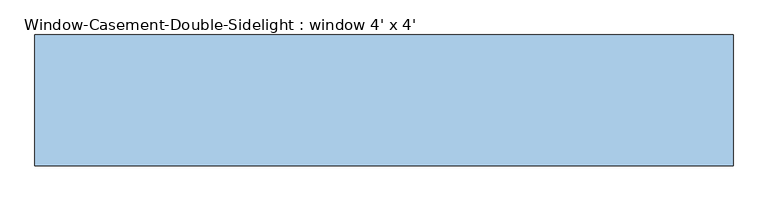
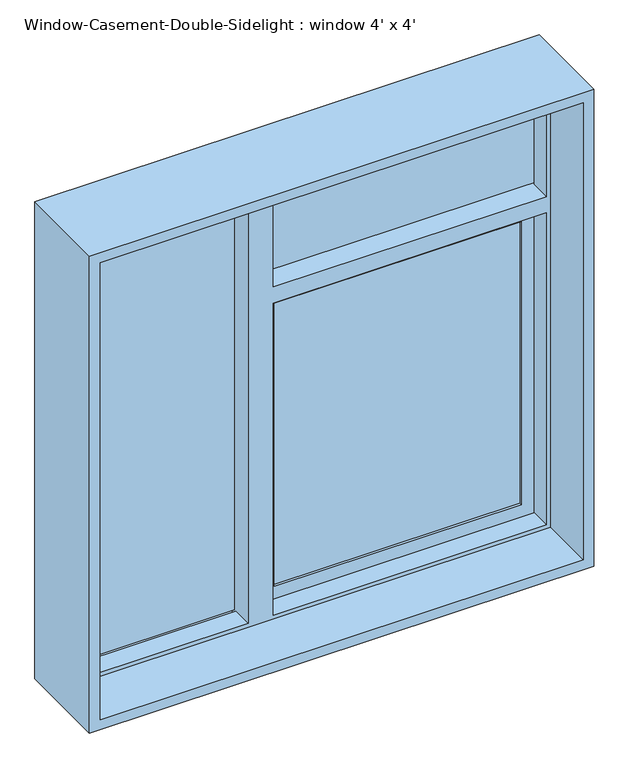
"""IFC4 building model written with IfcOpenShell, lengths in millimetres: window geometry, Window-Casement-Double-Sidelight : window 4' x 4'."""

from ifc_helpers import new_model, si_unit, frame, origin, place, context, project, spatial, polyline, outline, extrude, faceted_brep, source, transform, mapped, element, save


def window_casement_double_sidelight_window_4_x_4_2a492e8f(model_context):
    return source(origin(), model_context, "Body", "SolidModel", [
        extrude(outline(polyline([(542.3296875, 98.425), (-54.6496875, 98.425), (-54.6496875, 111.125), (542.3296875, 111.125), (542.3296875, 98.425)])), frame((0.0, 0.0, 981.6703125), z_axis=(0.0, 0.0, 1.0), x_axis=(1.0, 0.0, 0.0)), (0.0, 0.0, 1.0), 723.3642187),
        extrude(outline(polyline([(542.3296875, 85.725), (542.3296875, 79.375), (-54.6496875, 79.375), (-54.6496875, 85.725), (542.3296875, 85.725)])), frame((0.0, 0.0, 981.6703125), z_axis=(0.0, 0.0, 1.0), x_axis=(1.0, 0.0, 0.0)), (0.0, 0.0, 1.0), 723.3642187),
        extrude(outline(polyline([(-147.32, 98.425), (-147.32, 92.075), (-584.2, 92.075), (-584.2, 98.425), (-147.32, 98.425)])), frame((0.0, 0.0, 949.9203125), z_axis=(0.0, 0.0, 1.0), x_axis=(1.0, 0.0, 0.0)), (0.0, 0.0, 1.0), 1158.2796875),
        extrude(outline(polyline([(-147.32, 85.725), (-147.32, 79.375), (-584.2, 79.375), (-584.2, 85.725), (-147.32, 85.725)])), frame((0.0, 0.0, 949.9203125), z_axis=(0.0, 0.0, 1.0), x_axis=(1.0, 0.0, 0.0)), (0.0, 0.0, 1.0), 1158.2796875),
        extrude(outline(polyline([(584.2, 85.725), (584.2, 79.375), (-96.52, 79.375), (-96.52, 85.725), (584.2, 85.725)])), frame((0.0, 0.0, 1788.7751563), z_axis=(0.0, 0.0, 1.0), x_axis=(1.0, 0.0, 0.0)), (0.0, 0.0, 1.0), 319.4248438),
        extrude(outline(polyline([(584.2, 98.425), (584.2, 92.075), (-96.52, 92.075), (-96.52, 98.425), (584.2, 98.425)])), frame((0.0, 0.0, 1788.7751563), z_axis=(0.0, 0.0, 1.0), x_axis=(1.0, 0.0, 0.0)), (0.0, 0.0, 1.0), 319.4248438),
        faceted_brep([(-584.2, 73.025, 2108.2), (-584.2, 114.3, 2108.2), (584.2, 114.3, 2108.2), (584.2, 73.025, 2108.2), (-96.52, 73.025, 2108.2), (-96.52, 111.125, 2108.2), (-147.32, 111.125, 2108.2), (-147.32, 73.025, 2108.2), (-574.0796875, 22.225, 2098.0796875), (-574.0796875, 73.025, 2098.0796875), (-147.32, 73.025, 2098.0796875), (-147.32, 22.225, 2098.0796875), (574.0796875, 73.025, 2098.0796875), (574.0796875, 22.225, 2098.0796875), (-86.3996875, 22.225, 2098.0796875), (-86.3996875, 73.025, 2098.0796875), (-584.2, -114.3, 2108.2), (-584.2, 22.225, 2108.2), (584.2, 22.225, 2108.2), (584.2, -114.3, 2108.2), (-609.6, 114.3, 2133.6), (-609.6, -114.3, 2133.6), (609.6, -114.3, 2133.6), (609.6, 114.3, 2133.6), (584.2, 114.3, 939.8), (584.2, 73.025, 939.8), (584.2, 73.025, 1746.9048438), (584.2, 111.125, 1746.9048438), (584.2, 111.125, 1788.7751563), (584.2, 73.025, 1788.7751563), (574.0796875, 73.025, 1788.7751563), (574.0796875, 22.225, 1788.7751563), (574.0796875, 73.025, 949.9203125), (574.0796875, 22.225, 949.9203125), (574.0796875, 22.225, 1746.9048438), (574.0796875, 73.025, 1746.9048438), (584.2, 22.225, 939.8), (584.2, -114.3, 939.8), (609.6, -114.3, 914.4), (609.6, 114.3, 914.4), (-584.2, 114.3, 939.8), (-584.2, 73.025, 939.8), (-147.32, 73.025, 939.8), (-147.32, 111.125, 939.8), (-96.52, 111.125, 939.8), (-96.52, 73.025, 939.8), (-86.3996875, 73.025, 949.9203125), (-86.3996875, 22.225, 949.9203125), (-574.0796875, 73.025, 949.9203125), (-574.0796875, 22.225, 949.9203125), (-147.32, 22.225, 949.9203125), (-147.32, 73.025, 949.9203125), (-584.2, 22.225, 939.8), (-584.2, -114.3, 939.8), (-609.6, -114.3, 914.4), (-609.6, 114.3, 914.4), (-86.3996875, 73.025, 1788.7751563), (-96.52, 73.025, 1788.7751563), (-96.52, 73.025, 1746.9048438), (-86.3996875, 73.025, 1746.9048438), (-86.3996875, 22.225, 1788.7751563), (-86.3996875, 22.225, 1746.9048438), (-96.52, 111.125, 1788.7751563), (-96.52, 111.125, 1746.9048438)], [[[0, 1, 2, 3, 4, 5, 6, 7]], [[8, 9, 10, 11]], [[12, 13, 14, 15]], [[16, 17, 18, 19]], [[20, 21, 22, 23]], [[3, 2, 24, 25, 26, 27, 28, 29]], [[13, 12, 30, 31]], [[32, 33, 34, 35]], [[19, 18, 36, 37]], [[23, 22, 38, 39]], [[25, 24, 40, 41, 42, 43, 44, 45]], [[33, 32, 46, 47]], [[48, 49, 50, 51]], [[37, 36, 52, 53]], [[39, 38, 54, 55]], [[1, 0, 41, 40]], [[12, 15, 56, 57, 4, 3, 29, 30]], [[46, 32, 35, 26, 25, 45, 58, 59]], [[41, 0, 7, 10, 9, 48, 51, 42]], [[9, 8, 49, 48]], [[17, 52, 36, 18], [13, 31, 60, 14], [33, 47, 61, 34], [49, 8, 11, 50]], [[17, 16, 53, 52]], [[22, 21, 54, 38], [16, 19, 37, 53]], [[21, 20, 55, 54]], [[20, 23, 39, 55], [2, 1, 40, 24]], [[43, 6, 5, 62, 28, 27, 63, 44]], [[6, 43, 42, 51, 50, 11, 10, 7]], [[15, 14, 60, 56]], [[47, 46, 59, 61]], [[5, 4, 57, 62]], [[45, 44, 63, 58]], [[63, 27, 26, 35, 34, 61, 59, 58]], [[28, 62, 57, 56, 60, 31, 30, 29]]]),
        extrude(outline(polyline([(1746.9048438, 584.2), (1746.9048438, -96.52), (939.8, -96.52), (939.8, 584.2), (1746.9048438, 584.2)]), holes=[polyline([(981.6703125, 542.3296875), (981.6703125, -54.6496875), (1705.0345313, -54.6496875), (1705.0345313, 542.3296875), (981.6703125, 542.3296875)])]), frame((0.0, 73.025, 0.0), z_axis=(0.0, 1.0, 0.0), x_axis=(0.0, 0.0, 1.0)), (0.0, 0.0, 1.0), 31.75),
    ])


if __name__ == "__main__":
    model = new_model("IFC4")
    model_context = context("Model", 3, world=origin())
    ifc_project = project(units=[si_unit("LENGTHUNIT", "METRE", prefix="MILLI")], contexts=[model_context])
    site = spatial("IfcSite", under=ifc_project)
    building = spatial("IfcBuilding", under=site)
    placement = place(None, origin())
    window_casement_double_sidelight_window_4_x_4_shape = window_casement_double_sidelight_window_4_x_4_2a492e8f(model_context)
    element("IfcWindow", 1, ObjectType="Window-Casement-Double-Sidelight : window 4' x 4'", at=placement, inside=building, context=model_context, shape_type="MappedRepresentation", body=[
        mapped(window_casement_double_sidelight_window_4_x_4_shape, transform((0.0, 0.0, 0.0), x_axis=(1.0, 0.0, 0.0), y_axis=(0.0, 1.0, 0.0), z_axis=(0.0, 0.0, 1.0))),
    ])
    save(model, "model.ifc")

# Revit data of these elements
# Type "Window-Casement-Double-Sidelight : window 4' x 4'"
#   Type Mark = "22"
#   Fire Rating = "0.5h"
#   Assembly Code = "B2020100"
#   Analytic Construction = "Double glazing - domestic"
#   Window Inset [instance default] = 0' - 0 5/8"
#   Wall Thickness [instance default] = 0' - 6"
#   Visual Light Transmittance = 0.81
#   Transom Height Ratio = 0.3
#   Transom Height = 1' - 2.4"
#   Thermal Resistance (R) = 1.8146 (h·ft²·°F)/BTU
#   Solar Heat Gain Coefficient = 0.76
#   Side Width = 1' - 7.2"
#   Rough Width = 4' - 0 1/2"
#   Rough Height = 4' - 0 1/2"
#   Opening Window Width = 2' - 4.8"
#   Opening Window Height = 2' - 9.6"
#   Heat Transfer Coefficient (U) = 0.5511 BTU/(h·ft²·°F)
#   Height = 4' - 0"
#   Frame Gap 3 [instance default] = 0' - 1 83/128"
#   Frame Gap 2 [instance default] = 0' - 0 5/8"
#   Frame Gap 1 = 0' - 1 51/128"
#   Default Sill Height = 3' - 0"
#   Width = 4' - 0"
#   Frame Material = Metal - Aluminum
#   Glass Panel Material = Glass
#   Wall Closure = (empty or 0)
# Element 1 (IfcWindow, "Window-Casement-Double-Sidelight : window 4' x 4'")
#   Wall Thickness = 0' - 9"
#   Materials on its faces: "Metal - Aluminum", "Glass"
# Materials
#   "Metal - Aluminum": class "Metal", colour RGB 247 247 247, transparency 0
#   "Glass": class "Glass", colour RGB 0 128 192, transparency 0.75, Description = "Soda Lime Glass", Cost = 0
